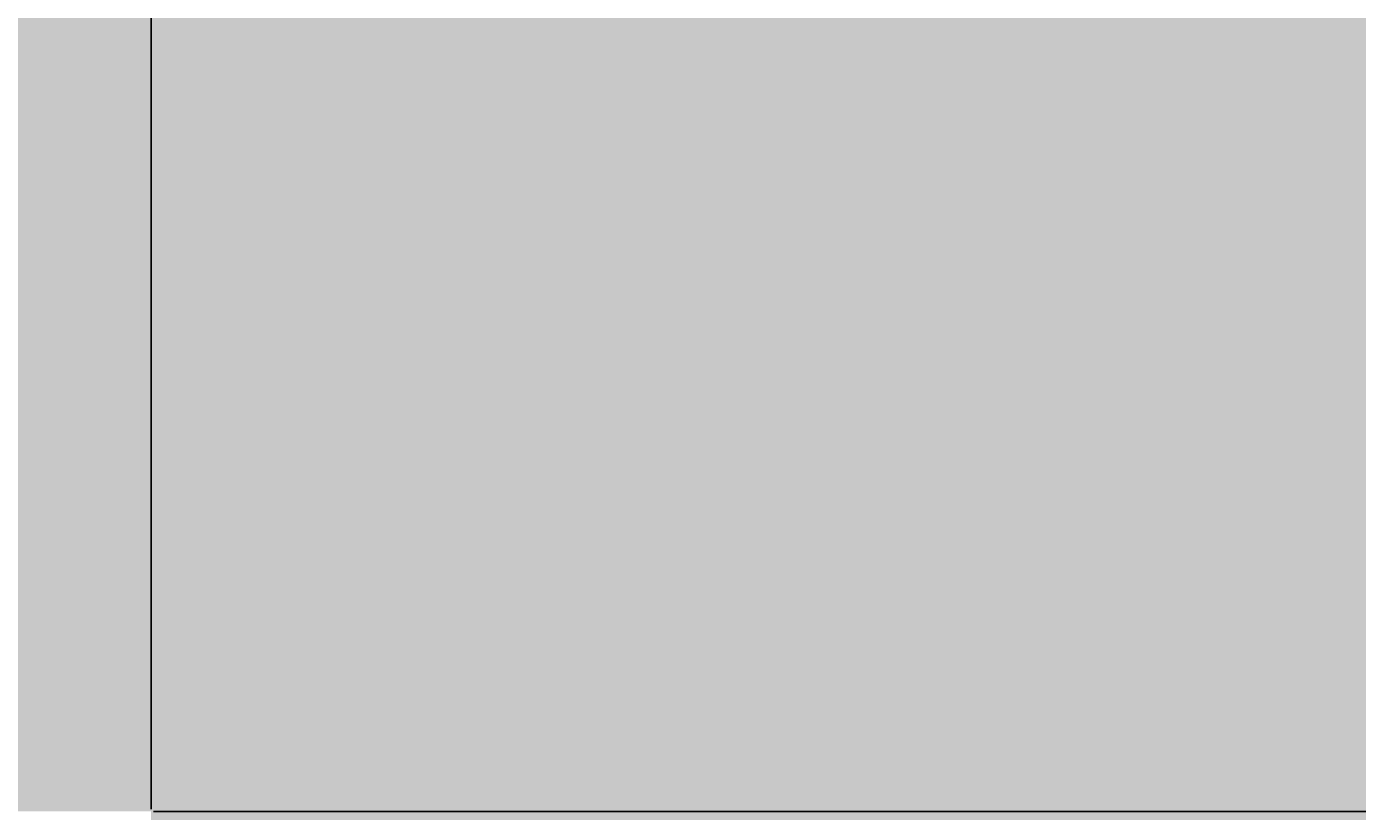
# Model space of a CAD drawing. Units: feet. Extents: x 2695 to 2912, y 795 to 1139.
# Tile 75 of 83: x 2840 to 2876, y 1021 to 1042. Entities that reach past the tile are written whole.
import ezdxf

# ---------------------------------------------------------------- set-up
doc = ezdxf.new("R2010")
doc.units = ezdxf.units.FT
doc.layers.add('A-ANNO-DIMS', color=2, linetype='Continuous', lineweight=18)
doc.layers.add('A-ELEV-PATT', color=252, linetype='Continuous', lineweight=13)
doc.styles.get("Standard").update_dxf_attribs({"font": 'arial.ttf'})
doc.dimstyles.get("Standard").update_dxf_attribs({"dimtxt": 0.18, "dimasz": 0.18, "dimexe": 0.18, "dimexo": 0.0625, "dimgap": 0.09, "dimtad": 0, "dimtih": 1, "dimtoh": 1, "dimdec": 1, "dimzin": 0, "dimdsep": 46, "dimlunit": 3, "dimtxsty": 'Standard', "dimcen": 0.09, "dimadec": 0, "dimazin": 0, "dimtfac": 1, "dimtdec": 1, "dimtofl": 0, "dimtmove": 0, "dimatfit": 3, "dimfxl": 1, "dimtolj": 1, "dimtzin": 0, "dimarcsym": 0})

# ---------------------------------------------------------------- blocks, each defined once
blk = doc.blocks.new('*D10')
at = {"layer": 'A-ANNO-DIMS', "color": 0, "lineweight": -2, "transparency": 16777216}
for p, q in [((2778.034, 1020.886), (2778.034, 1138.886)), ((2778.214, 1138.706), (2810.411, 1138.706)), ((2843.395, 1138.706), (2811.198, 1138.706)), ((2843.575, 1020.886), (2843.575, 1138.886))]:
    blk.add_line(p, q, dxfattribs=at)
at = {"layer": 'A-ANNO-DIMS', "color": 0, "transparency": 16777216}
for points in [[(2778.214, 1138.736), (2778.214, 1138.676), (2778.034, 1138.706)], [(2843.395, 1138.736), (2843.395, 1138.676), (2843.575, 1138.706)]]:
    blk.add_solid(points, dxfattribs=at)
at = {"layer": 'Defpoints', "color": 0, "transparency": 16777216}
for p in [(2843.575, 1138.706), (2778.034, 1020.824), (2843.575, 1020.824)]:
    blk.add_point(p, dxfattribs=at)
at = {"layer": 'A-ANNO-DIMS', "color": 0, "transparency": 16777216, "insert": (2810.805, 1138.706), "char_height": 0.18, "attachment_point": 5}
blk.add_mtext('\\A1;65.54', dxfattribs=at)
blk = doc.blocks.new('*D11')
at = {"layer": 'A-ANNO-DIMS', "color": 0, "lineweight": -2, "transparency": 16777216}
for p, q in [((2843.575, 1020.886), (2843.575, 1138.886)), ((2843.755, 1138.706), (2869.128, 1138.706)), ((2895.289, 1138.706), (2869.916, 1138.706)), ((2895.469, 1107.898), (2895.469, 1138.886))]:
    blk.add_line(p, q, dxfattribs=at)
at = {"layer": 'A-ANNO-DIMS', "color": 0, "transparency": 16777216}
for points in [[(2843.755, 1138.736), (2843.755, 1138.676), (2843.575, 1138.706)], [(2895.289, 1138.736), (2895.289, 1138.676), (2895.469, 1138.706)]]:
    blk.add_solid(points, dxfattribs=at)
at = {"layer": 'Defpoints', "color": 0, "transparency": 16777216}
for p in [(2895.469, 1138.706), (2895.469, 1107.835), (2843.575, 1020.824)]:
    blk.add_point(p, dxfattribs=at)
at = {"layer": 'A-ANNO-DIMS', "color": 0, "transparency": 16777216, "insert": (2869.522, 1138.706), "char_height": 0.18, "attachment_point": 5}
blk.add_mtext('\\A1;51.89', dxfattribs=at)
blk = doc.blocks.new('*D17')
at = {"layer": 'A-ANNO-DIMS', "color": 0, "lineweight": -2, "transparency": 16777216}
for p, q in [((2843.637, 1020.824), (2911.424, 1020.824)), ((2911.244, 1020.644), (2911.244, 979.059)), ((2911.244, 937.111), (2911.244, 978.695)), ((2890.699, 936.931), (2911.424, 936.931))]:
    blk.add_line(p, q, dxfattribs=at)
at = {"layer": 'A-ANNO-DIMS', "color": 0, "transparency": 16777216}
for points in [[(2911.214, 1020.644), (2911.274, 1020.644), (2911.244, 1020.824)], [(2911.214, 937.111), (2911.274, 937.111), (2911.244, 936.931)]]:
    blk.add_solid(points, dxfattribs=at)
at = {"layer": 'Defpoints', "color": 0, "transparency": 16777216}
for p in [(2843.575, 1020.824), (2911.244, 1020.824), (2890.636, 936.931)]:
    blk.add_point(p, dxfattribs=at)
at = {"layer": 'A-ANNO-DIMS', "color": 0, "transparency": 16777216, "insert": (2911.244, 978.877), "char_height": 0.18, "attachment_point": 5}
blk.add_mtext('\\A1;83.9', dxfattribs=at)
blk = doc.blocks.new('*D18')
at = {"layer": 'A-ANNO-DIMS', "color": 0, "lineweight": -2, "transparency": 16777216}
for p, q in [((2890.699, 1050.311), (2911.424, 1050.311)), ((2911.244, 1050.131), (2911.244, 1035.749)), ((2911.244, 1021.004), (2911.244, 1035.385)), ((2843.637, 1020.824), (2911.424, 1020.824))]:
    blk.add_line(p, q, dxfattribs=at)
at = {"layer": 'A-ANNO-DIMS', "color": 0, "transparency": 16777216}
for points in [[(2911.214, 1050.131), (2911.274, 1050.131), (2911.244, 1050.311)], [(2911.214, 1021.004), (2911.274, 1021.004), (2911.244, 1020.824)]]:
    blk.add_solid(points, dxfattribs=at)
at = {"layer": 'Defpoints', "color": 0, "transparency": 16777216}
for p in [(2890.636, 1050.311), (2911.244, 1050.311), (2843.575, 1020.824)]:
    blk.add_point(p, dxfattribs=at)
at = {"layer": 'A-ANNO-DIMS', "color": 0, "transparency": 16777216, "insert": (2911.244, 1035.567), "char_height": 0.18, "attachment_point": 5}
blk.add_mtext('\\A1;29.487', dxfattribs=at)
blk = doc.blocks.new('*D50')
at = {"layer": 'A-ANNO-DIMS', "color": 0, "lineweight": -2, "transparency": 16777216}
for p, q in [((2810.041, 972.03), (2810.041, 1138.886)), ((2810.221, 1138.706), (2848.721, 1138.706)), ((2888.008, 1138.706), (2849.508, 1138.706)), ((2888.188, 972.03), (2888.188, 1138.886))]:
    blk.add_line(p, q, dxfattribs=at)
at = {"layer": 'A-ANNO-DIMS', "color": 0, "transparency": 16777216}
for points in [[(2810.221, 1138.736), (2810.221, 1138.676), (2810.041, 1138.706)], [(2888.008, 1138.736), (2888.008, 1138.676), (2888.188, 1138.706)]]:
    blk.add_solid(points, dxfattribs=at)
at = {"layer": 'Defpoints', "color": 0, "transparency": 16777216}
for p in [(2888.188, 1138.706), (2810.041, 971.967), (2888.188, 971.967)]:
    blk.add_point(p, dxfattribs=at)
at = {"layer": 'A-ANNO-DIMS', "color": 0, "transparency": 16777216, "insert": (2849.114, 1138.706), "char_height": 0.18, "attachment_point": 5}
blk.add_mtext('\\A1;78.15', dxfattribs=at)

msp = doc.modelspace()

# ---------------------------------------------------------------- hatches: boundary and pattern name
at = {"layer": 'A-ELEV-PATT'}
h = msp.add_hatch(color=256, dxfattribs=at)
h.set_gradient(color1=(147, 149, 152), color2=(147, 149, 152), tint=1)
h.paths.add_polyline_path([(2770.6361, 1118.4096), (2710.6361, 1118.4096), (2710.6361, 1062.9306), (2770.6361, 1062.9306)])
h.paths.add_polyline_path([(2890.6361, 1103.3378), (2770.6361, 1103.3378), (2770.6361, 1062.9306), (2890.6361, 1062.9306)])
h.paths.add_polyline_path([(2730.7081, 1048.1052), (2755.1125, 1048.1052), (2755.1125, 936.9306), (2770.6361, 936.9306), (2770.6361, 1050.3105), (2715.8852, 1050.3105), (2715.8852, 936.9306), (2730.7081, 936.9306)])
h.paths.add_polyline_path([(2890.6361, 1050.3105), (2770.6361, 1050.3105), (2770.6361, 971.9673), (2778.0341, 971.9673), (2778.0341, 1020.8235), (2843.575, 1020.8235), (2843.575, 971.9673), (2890.6361, 971.9673)])
h.paths.add_polyline_path([(2888.1882, 970.7156), (2843.575, 970.7156), (2843.575, 964.8267), (2888.1882, 964.8267)])
h.paths.add_polyline_path([(2888.1882, 964.1328), (2843.575, 964.1328), (2843.575, 956.614), (2888.1882, 956.614)])
h.paths.add_polyline_path([(2888.1882, 955.9202), (2843.575, 955.9202), (2843.575, 949.2892), (2888.1882, 949.2892)])
h.paths.add_polyline_path([(2888.1882, 948.5954), (2843.575, 948.5954), (2843.575, 941.3507), (2888.1882, 941.3507)])
h.paths.add_polyline_path([(2888.1882, 940.6569), (2843.575, 940.6569), (2843.575, 936.9306), (2888.1882, 936.9306)])
h.paths.add_polyline_path([(2890.6361, 970.7156), (2888.9368, 970.7156), (2888.9368, 964.8267), (2890.6361, 964.8267)])
h.paths.add_polyline_path([(2890.6361, 964.1328), (2888.9368, 964.1328), (2888.9368, 956.614), (2890.6361, 956.614)])
h.paths.add_polyline_path([(2890.6361, 955.9202), (2888.9368, 955.9202), (2888.9368, 949.2892), (2890.6361, 949.2892)])
h.paths.add_polyline_path([(2890.6361, 940.6569), (2888.9368, 940.6569), (2888.9368, 936.9306), (2890.6361, 936.9306)])
h.paths.add_polyline_path([(2890.6361, 948.5954), (2888.9368, 948.5954), (2888.9368, 941.3507), (2890.6361, 941.3507)])
h.paths.add_polyline_path([(2772.5216, 970.7156), (2770.6361, 970.7156), (2770.6361, 964.8267), (2772.5216, 964.8267)])
h.paths.add_polyline_path([(2772.5216, 964.1328), (2770.6361, 964.1328), (2770.6361, 956.614), (2772.5216, 956.614)])
h.paths.add_polyline_path([(2772.5216, 955.9202), (2770.6361, 955.9202), (2770.6361, 949.2892), (2772.5216, 949.2892)])
h.paths.add_polyline_path([(2772.5216, 948.5954), (2770.6361, 948.5954), (2770.6361, 941.3507), (2772.5216, 941.3507)])
h.paths.add_polyline_path([(2772.5216, 940.6569), (2770.6361, 940.6569), (2770.6361, 936.9306), (2772.5216, 936.9306)])
h.paths.add_polyline_path([(2778.0341, 940.6569), (2773.2702, 940.6569), (2773.2702, 936.9306), (2778.0341, 936.9306)])
h.paths.add_polyline_path([(2778.0341, 970.7156), (2773.2702, 970.7156), (2773.2702, 964.8267), (2778.0341, 964.8267)])
h.paths.add_polyline_path([(2778.0341, 964.1328), (2773.2702, 964.1328), (2773.2702, 956.614), (2778.0341, 956.614)])
h.paths.add_polyline_path([(2778.0341, 955.9202), (2773.2702, 955.9202), (2773.2702, 949.2892), (2778.0341, 949.2892)])
h.paths.add_polyline_path([(2778.0341, 948.5954), (2773.2702, 948.5954), (2773.2702, 941.3507), (2778.0341, 941.3507)])
h.paths.add_polyline_path([(2810.0407, 940.6569), (2780.0341, 940.6569), (2780.0341, 936.9306), (2810.0407, 936.9306)])
h.paths.add_polyline_path([(2890.6361, 924.3105), (2770.6361, 924.3105), (2770.6361, 810.9306), (2773.5029, 810.9306), (2773.5029, 905.5143), (2805.9398, 905.5143), (2838.3767, 905.5143), (2838.3767, 810.9306), (2890.6361, 810.9306)])

# ---------------------------------------------------------------- dimensions: what is measured, and where the dimension line sits
at = {"layer": 'A-ANNO-DIMS'}
for base, p1, p2, picture, middle in [((2843.575, 1138.7056), (2778.0341, 1020.8235), (2843.575, 1020.8235), '*D10', (2810.8045, 1138.7056)), ((2888.1882, 1138.7056), (2810.0407, 971.9673), (2888.1882, 971.9673), '*D50', (2849.1144, 1138.7056)), ((2895.4694, 1138.7056), (2843.575, 1020.8235), (2895.4694, 1107.8352), '*D11', (2869.5222, 1138.7056))]:
    dim = msp.add_linear_dim(base=base, p1=p1, p2=p2, dimstyle='Standard', override={"dimdec": 2, "dimlfac": 1, "dimrnd": 0, "dimzin": 0, "dimdsep": 46, "dimlunit": 2}, dxfattribs=at)
    dim.commit()
    dim.dimension.update_dxf_attribs({"geometry": picture, "text_midpoint": middle})
for base, p1, p2, override, picture, middle in [((2911.2444, 1050.3105), (2843.575, 1020.8235), (2890.6361, 1050.3105), {"dimdec": 3, "dimlfac": 1, "dimrnd": 0, "dimzin": 0, "dimdsep": 46, "dimlunit": 2}, '*D18', (2911.2444, 1035.567)), ((2911.2444, 1020.8235), (2890.6361, 936.9306), (2843.575, 1020.8235), {"dimdec": 1, "dimlfac": 1, "dimrnd": 0, "dimzin": 0, "dimdsep": 46, "dimlunit": 2}, '*D17', (2911.2444, 978.877))]:
    dim = msp.add_linear_dim(base=base, p1=p1, p2=p2, angle=90, dimstyle='Standard', override=override, dxfattribs=at)
    dim.commit()
    dim.dimension.update_dxf_attribs({"geometry": picture, "text_midpoint": middle})

doc.saveas('drawing.dxf')
